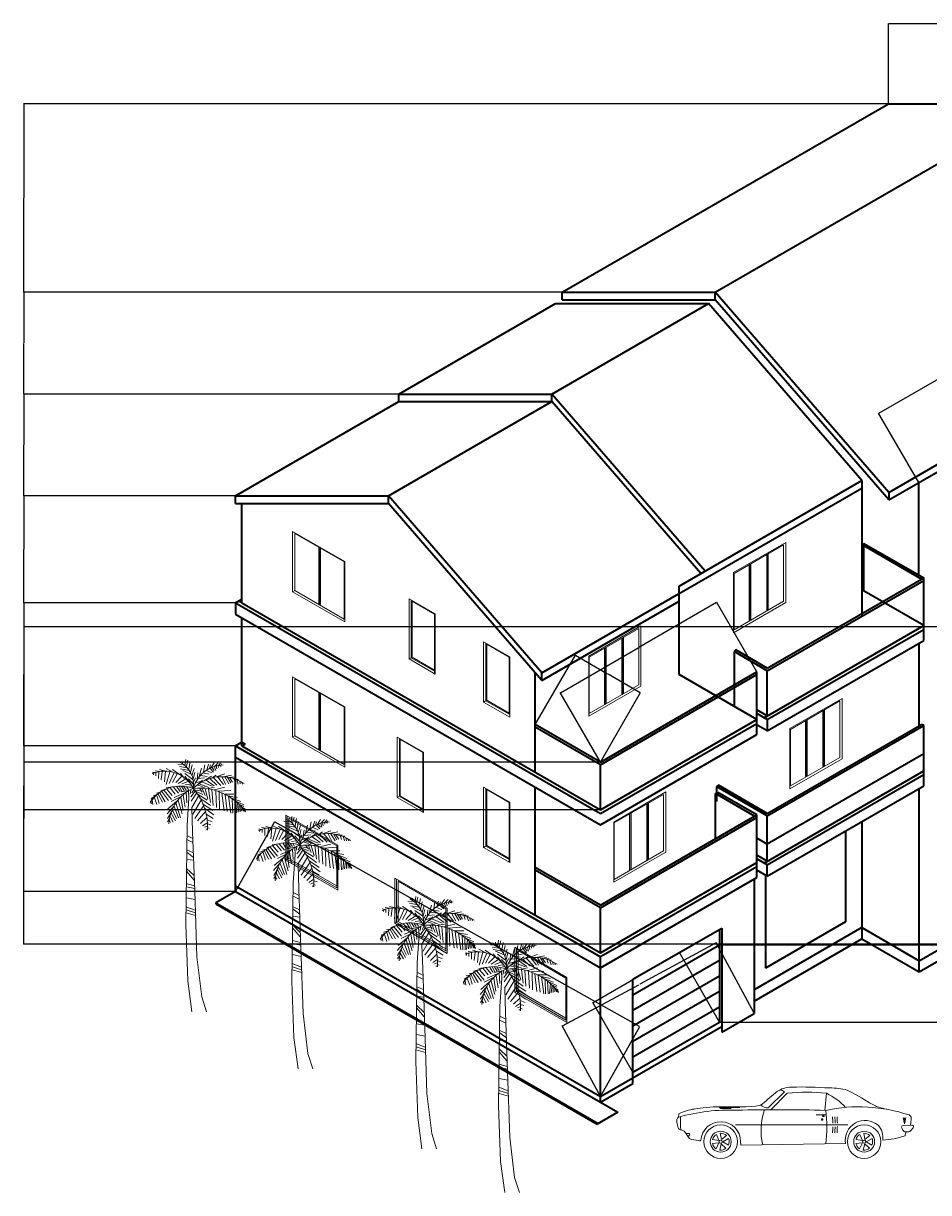
# Model space of a CAD drawing. Units: inches. Extents: x 159268 to 319465, y 115871 to 232488.
# Tile 1 of 2: x 159268 to 159989, y 115871 to 116803. Entities that reach past the tile are written whole.
import ezdxf

# ---------------------------------------------------------------- set-up
doc = ezdxf.new("R2010")
doc.units = ezdxf.units.IN
for name, color, linetype, lineweight in [('A-ANNO-DIMS', 2, 'Continuous', 18), ('A-ANNO-NPLT', 8, 'Continuous', 13), ('A-ELEV', 7, 'Continuous', 35), ('A-GLAZ', 4, 'Continuous', 18), ('C-SITE-VHCL', 8, 'Continuous', 13), ('L-PLNT', 3, 'Continuous', 13)]:
    doc.layers.add(name, color=color, linetype=linetype, lineweight=lineweight)
doc.styles.get("Standard").update_dxf_attribs({"font": 'arial.ttf'})
doc.dimstyles.get("Standard").update_dxf_attribs({"dimtxt": 0.18, "dimasz": 0.18, "dimexe": 0.18, "dimexo": 0.0625, "dimgap": 0.09, "dimtad": 0, "dimtih": 1, "dimtoh": 1, "dimdec": 4, "dimzin": 0, "dimdsep": 46, "dimtxsty": 'Standard', "dimcen": 0.09, "dimadec": 0, "dimazin": 0, "dimtfac": 1, "dimtdec": 4, "dimtofl": 0, "dimtmove": 0, "dimatfit": 3, "dimfxl": 1, "dimtolj": 1, "dimtzin": 0, "dimarcsym": 0})

# ---------------------------------------------------------------- blocks, each defined once
blk = doc.blocks.new('*U2')
for p, q in [((72.93, 40.23), (85.8, 53.18)), ((75, 38.82), (88.08, 51.97)), ((119.39, 51.91), (117.92, 38.32)), ((50.13, 41.06), (34.31, 40.98)), ((43.26, 39.85), (35.15, 39.78)), ((35.3, 40.46), (50.13, 40.62)), ((111.09, 34.73), (118.48, 34.64)), ((7.45, 19.78), (9.74, 19.8)), ((10.37, 19.19), (10.38, 18.56)), ((46.65, 26.83), (136.29, 26.77)), ((179.3, 24.35), (180.25, 22.49)), ((180.37, 26.17), (187.51, 26.41)), ((182.62, 21.14), (184.91, 21.28)), ((186.68, 22.17), (188.51, 24.37)), ((9.76, 17.93), (8.53, 17.92)), ((50.87, 13.52), (50.91, 10.52))]:
    blk.add_line(p, q)
for points in [[(35.31, 39.93), (35.3, 40.27, 0.269532), (35.14, 40.54), (34.38, 40.96, 0.575383), (34.15, 40.83), (34.15, 40.49, 0.269532), (34.32, 40.22), (35.08, 39.79, 0.575383)], [(28.49, 15.1), (33.61, 14.4), (31.65, 19.18, 0.199906)], [(34.64, 20.05), (35.56, 14.97), (39.5, 18.31, 0.199906)], [(142.85, 15.1), (147.96, 14.4), (146.01, 19.18, 0.199906)], [(148.99, 20.05), (149.91, 14.97), (153.85, 18.31, 0.199906)], [(31.31, 7.72), (33.55, 12.37), (28.4, 11.99, 0.199906)], [(39.19, 8.12), (35.46, 11.69), (34.23, 6.67, 0.199906)], [(41.25, 15.74), (36.7, 13.3), (41.09, 10.58, 0.199906)], [(145.66, 7.72), (147.9, 12.37), (142.75, 11.99, 0.199906)], [(153.54, 8.12), (149.81, 11.69), (148.59, 6.67, 0.199906)], [(155.6, 15.74), (151.06, 13.3), (155.45, 10.58, 0.199906)]]:
    blk.add_lwpolyline(points, format="xyb", close=True)
for points in [[(181.58, 27.46), (181.53, 31.95), (180.48, 32.43)], [(181.58, 27.46), (181.53, 31.95), (182.57, 32.45)], [(50.91, 10.52), (134.38, 11.83)]]:
    blk.add_lwpolyline(points)
for centre, radius in [((115.89, 31.01), 0.619), ((34.98, 13.35), 13.35), ((34.98, 13.35), 8.35), ((149.33, 13.35), 13.35), ((149.33, 13.35), 8.35), ((34.98, 13.35), 1.25), ((149.33, 13.35), 1.25)]:
    blk.add_circle(centre, radius)
for centre, radius, start, end in [((114.6, 105.09), 59.37, 237.61027, 240.97846), ((103.45, -95), 147.78, 83.81633, 95.97054), ((95.51, 3.91), 53.61, 43.27479, 63.56652), ((42.18, -111.35), 149.91, 87.83928, 105.80965), ((20.53, -3.15), 43.06, 98.53035, 116.11198), ((80.1, -1364.13), 1402.96, 88.42296, 91.3179), ((73.29, 50.49), 10.26, 230.42401, 268.00854), ((118.31, 22.51), 51.16, 161.43071, 193.23633), ((145.17, -84.88), 125.99, 71.52833, 102.12419), ((25.66, 24.94), 94.01, 351.8279, 8.16738), ((79.16, 30.11), 76.3, 177.57734, 185.52052), ((34.98, 13.35), 15.9, 0.63732, 176.34123), ((45.64, 26.83), 78.76, 0.85201, 4.65562), ((47.43, 26.85), 78.76, 0.85201, 4.65562), ((49.23, 26.87), 78.76, 0.85201, 4.65562), ((150.1, 14.36), 15.92, 49.2263, 189.1528), ((216.26, 37.76), 36.17, 188.46832, 196.53145), ((146.68, 36.98), 36.17, 344.74319, 352.80633), ((184.3, 32.25), 2.49, 357.93203, 71.52833), ((116.55, 34.7), 70.29, 353.19423, 357.93203), ((9.75, 19.18), 0.623, 0.63732, 90.63732), ((45.64, 26.83), 78.76, 355.26443, 358.86328), ((47.43, 26.85), 78.76, 355.26443, 358.86328), ((49.23, 26.87), 78.76, 355.26443, 358.86328), ((149.4, 16.55), 14.84, 352.72855, 41.66131), ((180.41, 24.92), 1.25, 91.93898, 207.10902), ((182.47, 23.63), 2.49, 207.10902, 273.46767), ((114.25, 37.03), 70.29, 344.3985, 346.93849), ((184.76, 23.76), 2.49, 273.46767, 320.16835), ((187.55, 25.16), 1.25, 320.16835, 91.93898), ((9.76, 18.55), 0.623, 270.63732, 0.63732), ((162.47, 70.82), 56.18, 271.6865, 290.2774)]:
    blk.add_arc(centre, radius, start, end)
blk.add_ellipse((116.89, 33.59), major_axis=(-0.63, -0.007), ratio=0.610043)
for points, knots in [([(11.39, 38.92), (18.06, 40.19), (30.91, 42.01), (64.77, 40.11), (70.25, 44.91), (82.35, 56.38), (99.18, 57.3), (116.06, 56.35), (133.04, 55.87), (145.24, 49.87), (153.62, 43.8), (161.17, 40.68), (164.92, 39.73), (167.29, 39.15)], [18.629823, 18.629823, 18.629823, 18.629823, 19.527405, 20.700571, 21.107983, 21.608568, 21.92336, 23.151359, 23.716171, 23.908743, 24.77794, 24.943072, 25.187755, 25.187755, 25.187755, 25.187755]), ([(19.11, 14.36), (18.99, 14.21), (18.5, 13.81), (15.35, 15), (9.19, 13.94), (7.26, 22.22), (3.01, 22.66), (1.32, 23.61), (0.64, 26.92), (-0.96, 31.49), (1.54, 32.64), (1.5, 34.06), (1.49, 34.8), (1.49, 35.06), (1.52, 35.3), (1.58, 35.51)], [16.815853, 16.815853, 16.815853, 16.815853, 16.838212, 16.885395, 17.18439, 17.479846, 17.654423, 17.670693, 17.696923, 18.016358, 18.052739, 18.140805, 18.140805, 18.140805, 18.172382, 18.172382, 18.172382, 18.172382])]:
    blk.add_open_spline(points, degree=3, knots=knots)
blk = doc.blocks.new('*U5')
for p, q in [((-6.727, 197.202), (-11.366, 197.45)), ((-7.5, 199.68), (-7.5, 197.946)), ((-5.567, 196.707), (-4.987, 201.167)), ((-4.407, 195.716), (-3.247, 200.672)), ((-2.474, 193.733), (-1.315, 199.433)), ((-1.121, 190.759), (0.232, 196.955)), ((9.317, 191.255), (10.283, 196.955)), ((11.829, 192.99), (13.182, 197.45)), ((13.956, 194.229), (14.729, 196.955)), ((15.116, 194.477), (17.822, 198.689)), ((18.015, 195.716), (20.914, 198.689)), ((19.368, 196.459), (19.948, 193.733)), ((20.914, 196.459), (21.301, 194.972)), ((21.301, 196.459), (22.847, 198.441)), ((22.074, 196.707), (23.427, 195.716)), ((23.234, 196.707), (23.62, 197.698)), ((-29.729, 190.759), (-31.469, 191.255)), ((-30.309, 190.512), (-30.695, 189.025)), ((-25.283, 191.751), (-29.342, 192.246)), ((-28.763, 190.759), (-28.763, 188.281)), ((-26.443, 191.503), (-26.636, 186.051)), ((-20.064, 191.751), (-25.863, 193.238)), ((-23.737, 191.751), (-24.51, 185.06)), ((-21.031, 191.998), (-21.804, 183.325)), ((-15.232, 191.255), (-20.644, 193.981)), ((-17.551, 191.503), (-20.451, 181.343)), ((-14.265, 190.759), (-18.131, 182.086)), ((-9.433, 189.025), (-15.618, 193.238)), ((-11.753, 189.768), (-15.425, 182.83)), ((-8.08, 188.034), (-12.912, 182.83)), ((-3.441, 194.477), (-10.013, 195.716)), ((-1.894, 192.494), (-9.24, 193.733)), ((-6.147, 186.299), (-9.24, 190.264)), ((-0.541, 189.52), (-7.307, 192.494)), ((-5.76, 190.016), (0.618, 185.308)), ((-5.76, 188.034), (-1.508, 182.582)), ((0.038, 188.281), (1.778, 193.981)), ((1.005, 185.803), (2.358, 190.759)), ((1.005, 182.582), (2.938, 186.547)), ((4.098, 185.06), (4.678, 190.512)), ((4.871, 186.051), (10.09, 186.547)), ((5.837, 187.786), (7.577, 194.229)), ((6.997, 188.529), (12.216, 187.786)), ((8.544, 190.512), (13.763, 189.52)), ((9.51, 184.317), (15.502, 188.034)), ((11.25, 192.494), (15.889, 190.512)), ((14.536, 193.981), (17.242, 191.255)), ((15.695, 186.299), (19.368, 188.777)), ((16.082, 194.972), (17.822, 192.494)), ((17.242, 186.547), (23.041, 180.599)), ((18.015, 195.468), (18.981, 192.494)), ((19.368, 187.29), (26.133, 189.768)), ((20.721, 187.042), (25.167, 181.343)), ((23.814, 187.29), (26.907, 181.343)), ((24.78, 187.538), (31.546, 188.777)), ((26.133, 187.29), (29.419, 181.838)), ((28.066, 187.29), (30.966, 182.582)), ((29.806, 186.795), (32.319, 183.078)), ((29.999, 186.795), (33.092, 187.29)), ((-21.031, 177.626), (-24.897, 176.387)), ((-15.618, 179.36), (-20.644, 178.617)), ((-20.064, 177.626), (-15.812, 172.67)), ((-17.358, 178.617), (-13.299, 173.661)), ((-15.038, 179.36), (-10.786, 174.404)), ((-12.332, 180.104), (-9.433, 175.643)), ((-4.987, 185.803), (-10.979, 182.086)), ((-10.206, 180.104), (-8.08, 175.891)), ((-8.273, 180.104), (-6.147, 176.635)), ((-3.247, 183.821), (-8.08, 181.838)), ((-6.34, 179.608), (-4.6, 177.13)), ((-1.315, 181.591), (-5.374, 181.095)), ((-4.021, 179.36), (-2.861, 177.378)), ((-2.668, 185.803), (1.198, 181.343)), ((-0.348, 180.352), (-1.894, 180.104)), ((1.585, 177.13), (0.038, 174.652)), ((1.585, 177.13), (6.61, 176.139)), ((2.938, 182.582), (6.61, 183.821)), ((4.098, 180.847), (8.35, 179.608)), ((4.871, 181.591), (8.544, 184.812)), ((5.644, 181.838), (13.569, 178.865)), ((6.224, 178.121), (8.157, 175.148)), ((7.384, 178.369), (10.476, 179.36)), ((7.77, 183.325), (16.082, 179.856)), ((8.157, 178.121), (10.476, 172.422)), ((10.476, 177.874), (12.796, 169.696)), ((11.25, 184.812), (17.628, 180.352)), ((11.829, 177.874), (18.015, 179.113)), ((13.182, 177.874), (14.729, 166.97)), ((14.536, 185.803), (19.948, 180.847)), ((15.889, 177.13), (16.855, 164.492)), ((18.015, 177.13), (26.133, 179.113)), ((32.512, 186.299), (35.218, 186.299)), ((33.479, 186.051), (34.445, 182.83)), ((35.605, 185.556), (37.151, 185.308)), ((35.798, 185.308), (36.958, 181.591)), ((38.118, 184.317), (38.504, 181.838)), ((39.857, 182.83), (40.244, 181.591)), ((-32.628, 167.961), (-33.208, 167.961)), ((-28.956, 172.174), (-32.435, 170.192)), ((-31.082, 169.944), (-32.435, 169.2)), ((-31.662, 168.705), (-31.082, 165.483)), ((-27.409, 173.413), (-30.695, 172.67)), ((-29.922, 170.687), (-27.989, 165.235)), ((-25.09, 175.148), (-28.376, 174.404)), ((-27.989, 172.422), (-26.056, 166.227)), ((-26.829, 173.661), (-23.544, 167.218)), ((-25.476, 174.652), (-21.224, 167.466)), ((-24.317, 175.891), (-18.711, 168.457)), ((-22.191, 176.635), (-16.391, 169.448)), ((-12.139, 167.961), (-19.098, 162.014)), ((-8.466, 171.678), (-16.585, 167.713)), ((-4.214, 175.148), (-14.072, 170.935)), ((-10.979, 168.457), (-7.887, 157.801)), ((-8.853, 170.935), (-7.113, 160.527)), ((-1.701, 176.882), (-8.66, 175.396)), ((-6.92, 172.917), (-5.374, 163.253)), ((-4.6, 174.9), (-4.021, 166.722)), ((-2.668, 176.387), (-2.376, 170.594)), ((-0.928, 176.882), (-1.508, 173.909)), ((2.551, 175.891), (-0.928, 171.431)), ((3.711, 174.404), (-0.541, 167.961)), ((5.257, 171.926), (-0.155, 163.005)), ((7.384, 168.705), (0.812, 157.553)), ((2.938, 175.891), (8.737, 173.413)), ((4.291, 173.909), (12.216, 168.953)), ((6.417, 170.439), (14.729, 164.492)), ((18.981, 175.891), (19.561, 163.005)), ((20.914, 175.891), (30.966, 176.635)), ((21.688, 175.396), (22.074, 161.518)), ((23.814, 174.404), (25.554, 160.279)), ((25.554, 173.661), (33.285, 173.661)), ((26.52, 173.165), (28.066, 159.784)), ((28.839, 172.174), (36.378, 170.687)), ((29.226, 171.926), (30.966, 158.545)), ((30.966, 170.687), (38.891, 167.713)), ((32.126, 169.696), (32.512, 158.545)), ((34.058, 168.705), (34.445, 158.545)), ((-32.628, 167.713), (-32.435, 165.979)), ((-14.265, 164.244), (-19.678, 158.049)), ((-16.005, 160.031), (-19.484, 154.084)), ((-16.585, 158.545), (-13.106, 152.35)), ((-15.618, 160.775), (-12.332, 154.332)), ((-14.265, 163.749), (-10.786, 154.828)), ((-12.719, 166.722), (-9.046, 154.828)), ((9.317, 164.244), (2.358, 154.332)), ((10.863, 159.784), (4.484, 152.35)), ((8.544, 165.979), (16.662, 160.527)), ((10.09, 162.51), (17.435, 157.058)), ((35.412, 167.713), (41.404, 164.988)), ((36.378, 166.474), (35.605, 158.792)), ((37.731, 165.235), (36.958, 159.288)), ((37.924, 165.235), (41.404, 163.749)), ((38.504, 164.492), (38.504, 159.536)), ((39.664, 163.253), (42.37, 161.766)), ((39.857, 162.757), (39.857, 160.031)), ((40.824, 161.766), (41.21, 160.031)), ((41.21, 161.518), (42.757, 160.279)), ((-18.131, 153.589), (-19.484, 151.606)), ((-17.938, 152.597), (-16.972, 151.111)), ((-17.358, 155.819), (-14.845, 151.358)), ((11.829, 155.075), (6.804, 150.119)), ((12.603, 151.111), (8.544, 148.385)), ((11.443, 157.553), (16.855, 154.332)), ((12.216, 153.093), (16.082, 151.606)), ((12.603, 149.872), (15.116, 149.128)), ((-4.081, 140.645), (0.753, 138.261)), ((12.216, 148.137), (10.09, 147.393)), ((12.409, 145.659), (11.056, 145.659)), ((12.409, 146.898), (13.763, 146.402)), ((-4.081, 137.547), (0.753, 135.163)), ((-4.081, 129.205), (1.124, 126.821)), ((-4.081, 127.298), (1.31, 123.246)), ((-4.081, 121.578), (1.31, 120.863)), ((-4.453, 112.283), (1.682, 105.133)), ((-4.267, 114.428), (1.682, 108.708)), ((-4.639, 102.273), (1.868, 100.604)), ((-4.453, 99.651), (2.24, 98.459)), ((-4.825, 83.921), (2.612, 81.061)), ((-4.453, 91.071), (2.426, 89.641)), ((-4.639, 81.299), (2.797, 78.916)), ((-4.639, 78.916), (2.797, 76.771))]:
    blk.add_line(p, q)
for points in [[(-2.363, 170.553), (-3.88, 148.505), (-4.988, 69.634), (-3.325, 24.869), (0, 0)], [(-0.116, 162.848), (0.554, 143.532), (2.217, 96.635), (3.88, 44.054), (7.76, 12.079), (11.64, 0)]]:
    blk.add_lwpolyline(points)
for centre, radius, start, end in [((-18.427, 181.448), 19.715, 350.285, 64.11229), ((25.595, 171.567), 25.395, 91.40319, 163.882), ((-21.738, 166.094), 25.899, 27.67115, 112.5305), ((23.687, 155.341), 32.188, 56.19272, 134.3213), ((-9.259, 151.732), 28.386, 68.38311, 147.5322), ((14.394, 148.393), 32.752, 113.7592, 177.4133), ((5.828, 132.718), 45.639, 35.98777, 95.82273), ((-32.8, 147.923), 45.309, 356.1943, 41.37848)]:
    blk.add_arc(centre, radius, start, end)
blk = doc.blocks.new('WIN-GROUND')
for p, q in [((159476.63, 116172), (159518.2, 116148)), ((159476.63, 116136), (159476.63, 116172)), ((159477.91, 116136.72), (159477.91, 116171.27)), ((159479.23, 116137.5), (159479.23, 116169.5)), ((159479.23, 116169.5), (159517.33, 116147.5)), ((159517.33, 116147.5), (159517.33, 116113.96)), ((159518.2, 116148), (159518.2, 116112)), ((159476.63, 116136), (159479.23, 116137.5)), ((159517.33, 116115.5), (159479.23, 116137.5)), ((159518.2, 116112), (159476.63, 116136)), ((159517.33, 116113.96), (159477.91, 116136.72))]:
    blk.add_line(p, q)
blk = doc.blocks.new('WIN-NARROW')
for p, q in [((159565.58, 116186), (159565.58, 116234)), ((159565.58, 116234), (159586.37, 116222)), ((159567.31, 116187), (159567.31, 116233)), ((159568.02, 116187.41), (159568.02, 116232.1)), ((159568.02, 116232.1), (159585.93, 116221.75)), ((159585.93, 116221.75), (159585.93, 116174.25)), ((159586.37, 116222), (159586.37, 116174)), ((159565.58, 116186), (159568.02, 116187.41)), ((159586.37, 116174), (159565.58, 116186)), ((159586.37, 116176), (159567.31, 116187)), ((159586.37, 116176.82), (159568.02, 116187.41))]:
    blk.add_line(p, q)
blk = doc.blocks.new('WIN-2PANE')
for p, q in [((159482.18, 116234.16), (159482.18, 116282.16)), ((159482.18, 116282.16), (159523.75, 116258.16)), ((159483.91, 116235.16), (159483.91, 116280.66)), ((159483.91, 116280.66), (159523.75, 116257.66)), ((159502.97, 116269.66), (159502.97, 116224.16)), ((159503.83, 116269.16), (159503.83, 116223.66)), ((159504.26, 116268.91), (159504.26, 116223.91)), ((159523.32, 116258.41), (159523.32, 116212.41)), ((159523.75, 116258.16), (159523.75, 116210.16)), ((159482.18, 116234.16), (159483.91, 116235.16)), ((159523.75, 116210.16), (159482.18, 116234.16)), ((159523.32, 116212.41), (159483.91, 116235.16)), ((159503.83, 116223.66), (159504.26, 116223.91))]:
    blk.add_line(p, q)
blk = doc.blocks.new('WIN-3PANE')
for p, q in [((159718.21, 116298.71), (159759.78, 116322.71)), ((159718.64, 116297.96), (159758.05, 116320.71)), ((159758.05, 116320.71), (159758.05, 116275.71)), ((159759.78, 116322.71), (159759.78, 116274.71)), ((159731.2, 116260.21), (159731.2, 116305.21)), ((159732.07, 116260.71), (159732.07, 116305.71)), ((159744.62, 116268.46), (159744.62, 116312.96)), ((159745.06, 116268.21), (159745.06, 116313.21)), ((159745.92, 116268.71), (159745.92, 116313.71)), ((159718.21, 116250.71), (159718.21, 116298.71)), ((159718.64, 116252.96), (159718.64, 116297.96)), ((159730.77, 116260.46), (159730.77, 116304.96)), ((159759.78, 116274.71), (159718.21, 116250.71)), ((159758.05, 116275.71), (159718.64, 116252.96)), ((159744.62, 116268.46), (159745.06, 116268.21)), ((159730.77, 116260.46), (159731.2, 116260.21))]:
    blk.add_line(p, q)
blk = doc.blocks.new('*D10')
at = {"layer": 'A-ANNO-DIMS', "color": 0, "lineweight": -2, "transparency": 16777216}
for p, q in [((159436.46, 116227.11), (159267.73, 116227.11)), ((159267.91, 116226.93), (159267.91, 116169.29)), ((159267.91, 116111.29), (159267.91, 116168.93)), ((159436.46, 116111.11), (159267.73, 116111.11))]:
    blk.add_line(p, q, dxfattribs=at)
at = {"layer": 'A-ANNO-DIMS', "color": 0, "transparency": 16777216}
for points in [[(159267.88, 116226.93), (159267.94, 116226.93), (159267.91, 116227.11)], [(159267.88, 116111.29), (159267.94, 116111.29), (159267.91, 116111.11)]]:
    blk.add_solid(points, dxfattribs=at)
at = {"layer": 'Defpoints', "color": 0, "transparency": 16777216}
for p in [(159267.91, 116227.11), (159436.52, 116227.11), (159436.52, 116111.11)]:
    blk.add_point(p, dxfattribs=at)
at = {"layer": 'A-ANNO-DIMS', "color": 0, "transparency": 16777216, "insert": (159267.91, 116169.11), "char_height": 0.18, "attachment_point": 5}
blk.add_mtext('\\A1;116', dxfattribs=at)
blk = doc.blocks.new('*D11')
at = {"layer": 'A-ANNO-DIMS', "color": 0, "lineweight": -2, "transparency": 16777216}
for p, q in [((159436.46, 116341.11), (159267.73, 116341.11)), ((159267.91, 116340.93), (159267.91, 116284.29)), ((159267.91, 116227.29), (159267.91, 116283.93)), ((159436.46, 116227.11), (159267.73, 116227.11))]:
    blk.add_line(p, q, dxfattribs=at)
at = {"layer": 'A-ANNO-DIMS', "color": 0, "transparency": 16777216}
for points in [[(159267.88, 116340.93), (159267.94, 116340.93), (159267.91, 116341.11)], [(159267.88, 116227.29), (159267.94, 116227.29), (159267.91, 116227.11)]]:
    blk.add_solid(points, dxfattribs=at)
at = {"layer": 'Defpoints', "color": 0, "transparency": 16777216}
for p in [(159267.91, 116341.11), (159436.52, 116341.11), (159436.52, 116227.11)]:
    blk.add_point(p, dxfattribs=at)
at = {"layer": 'A-ANNO-DIMS', "color": 0, "transparency": 16777216, "insert": (159267.91, 116284.11), "char_height": 0.18, "attachment_point": 5}
blk.add_mtext('\\A1;114', dxfattribs=at)
blk = doc.blocks.new('*D12')
at = {"layer": 'A-ANNO-DIMS', "color": 0, "lineweight": -2, "transparency": 16777216}
for p, q in [((159436.46, 116426.35), (159267.73, 116426.35)), ((159267.91, 116426.17), (159267.91, 116383.91)), ((159267.91, 116341.29), (159267.91, 116383.55)), ((159436.46, 116341.11), (159267.73, 116341.11))]:
    blk.add_line(p, q, dxfattribs=at)
at = {"layer": 'A-ANNO-DIMS', "color": 0, "transparency": 16777216}
for points in [[(159267.88, 116426.17), (159267.94, 116426.17), (159267.91, 116426.35)], [(159267.88, 116341.29), (159267.94, 116341.29), (159267.91, 116341.11)]]:
    blk.add_solid(points, dxfattribs=at)
at = {"layer": 'Defpoints', "color": 0, "transparency": 16777216}
for p in [(159267.91, 116426.35), (159436.52, 116426.35), (159436.52, 116341.11)]:
    blk.add_point(p, dxfattribs=at)
at = {"layer": 'A-ANNO-DIMS', "color": 0, "transparency": 16777216, "insert": (159267.91, 116383.73), "char_height": 0.18, "attachment_point": 5}
blk.add_mtext('\\A1;85.24', dxfattribs=at)
blk = doc.blocks.new('*D13')
at = {"layer": 'A-ANNO-DIMS', "color": 0, "lineweight": -2, "transparency": 16777216}
for p, q in [((159566.67, 116507.53), (159267.73, 116507.53)), ((159267.91, 116507.35), (159267.91, 116467.12)), ((159267.91, 116426.53), (159267.91, 116466.76)), ((159436.46, 116426.35), (159267.73, 116426.35))]:
    blk.add_line(p, q, dxfattribs=at)
at = {"layer": 'A-ANNO-DIMS', "color": 0, "transparency": 16777216}
for points in [[(159267.88, 116507.35), (159267.94, 116507.35), (159267.91, 116507.53)], [(159267.88, 116426.53), (159267.94, 116426.53), (159267.91, 116426.35)]]:
    blk.add_solid(points, dxfattribs=at)
at = {"layer": 'Defpoints', "color": 0, "transparency": 16777216}
for p in [(159267.91, 116507.53), (159566.74, 116507.53), (159436.52, 116426.35)]:
    blk.add_point(p, dxfattribs=at)
at = {"layer": 'A-ANNO-DIMS', "color": 0, "transparency": 16777216, "insert": (159267.91, 116466.94), "char_height": 0.18, "attachment_point": 5}
blk.add_mtext('\\A1;81.18', dxfattribs=at)
blk = doc.blocks.new('*D14')
at = {"layer": 'A-ANNO-DIMS', "color": 0, "lineweight": -2, "transparency": 16777216}
for p, q in [((159696.94, 116588.74), (159267.73, 116588.74)), ((159267.91, 116588.56), (159267.91, 116548.31)), ((159267.91, 116507.71), (159267.91, 116547.95)), ((159566.67, 116507.53), (159267.73, 116507.53))]:
    blk.add_line(p, q, dxfattribs=at)
at = {"layer": 'A-ANNO-DIMS', "color": 0, "transparency": 16777216}
for points in [[(159267.88, 116588.56), (159267.94, 116588.56), (159267.91, 116588.74)], [(159267.88, 116507.71), (159267.94, 116507.71), (159267.91, 116507.53)]]:
    blk.add_solid(points, dxfattribs=at)
at = {"layer": 'Defpoints', "color": 0, "transparency": 16777216}
for p in [(159267.91, 116588.74), (159697, 116588.74), (159566.74, 116507.53)]:
    blk.add_point(p, dxfattribs=at)
at = {"layer": 'A-ANNO-DIMS', "color": 0, "transparency": 16777216, "insert": (159267.91, 116548.13), "char_height": 0.18, "attachment_point": 5}
blk.add_mtext('\\A1;81.2', dxfattribs=at)
blk = doc.blocks.new('*D15')
at = {"layer": 'A-ANNO-DIMS', "color": 0, "lineweight": -2, "transparency": 16777216}
for p, q in [((159957.23, 116739.02), (159267.73, 116739.02)), ((159267.91, 116738.84), (159267.91, 116664.06)), ((159267.91, 116588.92), (159267.91, 116663.69)), ((159696.94, 116588.74), (159267.73, 116588.74))]:
    blk.add_line(p, q, dxfattribs=at)
at = {"layer": 'A-ANNO-DIMS', "color": 0, "transparency": 16777216}
for points in [[(159267.88, 116738.84), (159267.94, 116738.84), (159267.91, 116739.02)], [(159267.88, 116588.92), (159267.94, 116588.92), (159267.91, 116588.74)]]:
    blk.add_solid(points, dxfattribs=at)
at = {"layer": 'Defpoints', "color": 0, "transparency": 16777216}
for p in [(159267.91, 116739.02), (159957.3, 116739.02), (159697, 116588.74)]:
    blk.add_point(p, dxfattribs=at)
at = {"layer": 'A-ANNO-DIMS', "color": 0, "transparency": 16777216, "insert": (159267.91, 116663.88), "char_height": 0.18, "attachment_point": 5}
blk.add_mtext('\\A1;150.28', dxfattribs=at)
blk = doc.blocks.new('*D16')
at = {"layer": 'A-ANNO-DIMS', "color": 0, "lineweight": -2, "transparency": 16777216}
for p, q in [((159436.55, 116111.16), (159467.88, 116166.93)), ((159467.95, 116166.69), (159612.96, 116085.21)), ((159758.62, 116003.36), (159613.61, 116084.84)), ((159727.53, 115947.66), (159758.87, 116003.43))]:
    blk.add_line(p, q, dxfattribs=at)
at = {"layer": 'A-ANNO-DIMS', "color": 0, "transparency": 16777216}
for points in [[(159467.97, 116166.71), (159467.94, 116166.66), (159467.8, 116166.77)], [(159758.64, 116003.39), (159758.61, 116003.34), (159758.78, 116003.27)]]:
    blk.add_solid(points, dxfattribs=at)
at = {"layer": 'Defpoints', "color": 0, "transparency": 16777216}
for p in [(159436.52, 116111.11), (159758.78, 116003.27), (159727.5, 115947.61)]:
    blk.add_point(p, dxfattribs=at)
at = {"layer": 'A-ANNO-DIMS', "color": 0, "transparency": 16777216, "insert": (159613.29, 116085.02), "char_height": 0.18, "attachment_point": 5}
blk.add_mtext('\\A1;333.8', dxfattribs=at)
blk = doc.blocks.new('*D17')
at = {"layer": 'A-ANNO-DIMS', "color": 0, "lineweight": -2, "transparency": 16777216}
for p, q in [((159819.67, 116070.02), (159758.82, 116037.12)), ((159850.16, 116014), (159819.74, 116070.27)), ((159697.29, 116003.86), (159758.14, 116036.76)), ((159727.47, 115947.66), (159697.05, 116003.93))]:
    blk.add_line(p, q, dxfattribs=at)
at = {"layer": 'A-ANNO-DIMS', "color": 0, "transparency": 16777216}
for points in [[(159819.65, 116070.05), (159819.68, 116070), (159819.82, 116070.11)], [(159697.28, 116003.89), (159697.31, 116003.84), (159697.14, 116003.78)]]:
    blk.add_solid(points, dxfattribs=at)
at = {"layer": 'Defpoints', "color": 0, "transparency": 16777216}
for p in [(159819.82, 116070.11), (159850.19, 116013.94), (159727.5, 115947.61)]:
    blk.add_point(p, dxfattribs=at)
at = {"layer": 'A-ANNO-DIMS', "color": 0, "transparency": 16777216, "insert": (159758.48, 116036.94), "char_height": 0.18, "attachment_point": 5}
blk.add_mtext('\\A1;139.47', dxfattribs=at)
blk = doc.blocks.new('*D18')
at = {"layer": 'A-ANNO-DIMS', "color": 0, "lineweight": -2, "transparency": 16777216}
for p, q in [((159790.4, 116062.15), (159756.37, 116042.5)), ((159822.45, 116007), (159790.46, 116062.4)), ((159721.71, 116022.5), (159755.74, 116042.14)), ((159753.45, 115967.16), (159721.47, 116022.56))]:
    blk.add_line(p, q, dxfattribs=at)
at = {"layer": 'A-ANNO-DIMS', "color": 0, "transparency": 16777216}
for points in [[(159790.38, 116062.18), (159790.41, 116062.12), (159790.55, 116062.24)], [(159721.7, 116022.52), (159721.73, 116022.47), (159721.56, 116022.41)]]:
    blk.add_solid(points, dxfattribs=at)
at = {"layer": 'Defpoints', "color": 0, "transparency": 16777216}
for p in [(159790.55, 116062.24), (159822.48, 116006.94), (159753.48, 115967.11)]:
    blk.add_point(p, dxfattribs=at)
at = {"layer": 'A-ANNO-DIMS', "color": 0, "transparency": 16777216, "insert": (159756.06, 116042.32), "char_height": 0.18, "attachment_point": 5}
blk.add_mtext('\\A1;79.67', dxfattribs=at)
blk = doc.blocks.new('*D19')
at = {"layer": 'A-ANNO-DIMS', "color": 0, "lineweight": -2, "transparency": 16777216}
for p, q in [((159822.54, 116068.59), (160661.48, 116068.59)), ((160661.3, 116068.41), (160661.3, 116037.95)), ((160661.3, 116007.12), (160661.3, 116037.59)), ((159822.54, 116006.94), (160661.48, 116006.94))]:
    blk.add_line(p, q, dxfattribs=at)
at = {"layer": 'A-ANNO-DIMS', "color": 0, "transparency": 16777216}
for points in [[(160661.27, 116068.41), (160661.33, 116068.41), (160661.3, 116068.59)], [(160661.27, 116007.12), (160661.33, 116007.12), (160661.3, 116006.94)]]:
    blk.add_solid(points, dxfattribs=at)
at = {"layer": 'Defpoints', "color": 0, "transparency": 16777216}
for p in [(159822.48, 116068.59), (160661.3, 116068.59), (159822.48, 116006.94)]:
    blk.add_point(p, dxfattribs=at)
at = {"layer": 'A-ANNO-DIMS', "color": 0, "transparency": 16777216, "insert": (160661.3, 116037.77), "char_height": 0.18, "attachment_point": 5}
blk.add_mtext('\\A1;61.65', dxfattribs=at)
blk = doc.blocks.new('*D20')
at = {"layer": 'A-ANNO-DIMS', "color": 0, "lineweight": -2, "transparency": 16777216}
for p, q in [((160177.25, 116623.87), (160063.72, 116558.33)), ((160209.3, 116568.72), (160177.32, 116624.12)), ((159949.55, 116492.41), (160063.09, 116557.96)), ((159981.29, 116437.08), (159949.31, 116492.48))]:
    blk.add_line(p, q, dxfattribs=at)
at = {"layer": 'A-ANNO-DIMS', "color": 0, "transparency": 16777216}
for points in [[(160177.23, 116623.9), (160177.26, 116623.85), (160177.41, 116623.96)], [(159949.54, 116492.44), (159949.57, 116492.39), (159949.4, 116492.32)]]:
    blk.add_solid(points, dxfattribs=at)
at = {"layer": 'Defpoints', "color": 0, "transparency": 16777216}
for p in [(160177.41, 116623.96), (160209.33, 116568.67), (159981.32, 116437.03)]:
    blk.add_point(p, dxfattribs=at)
at = {"layer": 'A-ANNO-DIMS', "color": 0, "transparency": 16777216, "insert": (160063.4, 116558.14), "char_height": 0.18, "attachment_point": 5}
blk.add_mtext('\\A1;263.3', dxfattribs=at)
blk = doc.blocks.new('*D22')
at = {"layer": 'A-ANNO-DIMS', "color": 0, "lineweight": -2, "transparency": 16777216}
for p, q in [((160024.97, 116321.98), (159267.73, 116321.98)), ((159267.91, 116321.8), (159267.91, 116195.69)), ((159267.91, 116069.21), (159267.91, 116195.33)), ((160024.97, 116069.03), (159267.73, 116069.03))]:
    blk.add_line(p, q, dxfattribs=at)
at = {"layer": 'A-ANNO-DIMS', "color": 0, "transparency": 16777216}
for points in [[(159267.88, 116321.8), (159267.94, 116321.8), (159267.91, 116321.98)], [(159267.88, 116069.21), (159267.94, 116069.21), (159267.91, 116069.03)]]:
    blk.add_solid(points, dxfattribs=at)
at = {"layer": 'Defpoints', "color": 0, "transparency": 16777216}
for p in [(159267.91, 116321.98), (160025.03, 116321.98), (160025.03, 116069.03)]:
    blk.add_point(p, dxfattribs=at)
at = {"layer": 'A-ANNO-DIMS', "color": 0, "transparency": 16777216, "insert": (159267.91, 116195.51), "char_height": 0.18, "attachment_point": 5}
blk.add_mtext('\\A1;252.95', dxfattribs=at)
blk = doc.blocks.new('*D31')
at = {"layer": 'A-ANNO-DIMS', "color": 0, "lineweight": -2, "transparency": 16777216}
for p, q in [((159820.13, 116341.32), (159758.21, 116305.57)), ((159852.18, 116286.16), (159820.2, 116341.56)), ((159695.73, 116269.5), (159757.65, 116305.24)), ((159727.47, 116214.16), (159695.49, 116269.56))]:
    blk.add_line(p, q, dxfattribs=at)
at = {"layer": 'A-ANNO-DIMS', "color": 0, "transparency": 16777216}
for points in [[(159820.12, 116341.34), (159820.15, 116341.29), (159820.29, 116341.41)], [(159695.72, 116269.52), (159695.75, 116269.47), (159695.58, 116269.41)]]:
    blk.add_solid(points, dxfattribs=at)
at = {"layer": 'Defpoints', "color": 0, "transparency": 16777216}
for p in [(159820.29, 116341.41), (159852.21, 116286.11), (159727.5, 116214.11)]:
    blk.add_point(p, dxfattribs=at)
at = {"layer": 'A-ANNO-DIMS', "color": 0, "transparency": 16777216, "insert": (159757.93, 116305.41), "char_height": 0.18, "attachment_point": 5}
blk.add_mtext('\\A1;144', dxfattribs=at)
blk = doc.blocks.new('*D32')
at = {"layer": 'A-ANNO-DIMS', "color": 0, "lineweight": -2, "transparency": 16777216}
for p, q in [((159675.57, 116244.16), (159707.56, 116299.56)), ((159707.62, 116299.32), (159733.23, 116284.53)), ((159759.27, 116269.5), (159733.67, 116284.28)), ((159727.53, 116214.16), (159759.52, 116269.56))]:
    blk.add_line(p, q, dxfattribs=at)
at = {"layer": 'A-ANNO-DIMS', "color": 0, "transparency": 16777216}
for points in [[(159707.64, 116299.34), (159707.61, 116299.29), (159707.47, 116299.41)], [(159759.29, 116269.52), (159759.26, 116269.47), (159759.43, 116269.41)]]:
    blk.add_solid(points, dxfattribs=at)
at = {"layer": 'Defpoints', "color": 0, "transparency": 16777216}
for p in [(159759.43, 116269.41), (159675.54, 116244.11), (159727.5, 116214.11)]:
    blk.add_point(p, dxfattribs=at)
at = {"layer": 'A-ANNO-DIMS', "color": 0, "transparency": 16777216, "insert": (159733.45, 116284.41), "char_height": 0.18, "attachment_point": 5}
blk.add_mtext('\\A1;60', dxfattribs=at)
blk = doc.blocks.new('*D33')
at = {"layer": 'A-ANNO-DIMS', "color": 0, "lineweight": -2, "transparency": 16777216}
for p, q in [((159727.44, 116214.11), (159267.73, 116214.11)), ((159267.91, 116213.93), (159267.91, 116195.29)), ((159267.91, 116176.29), (159267.91, 116194.93)), ((159727.44, 116176.11), (159267.73, 116176.11))]:
    blk.add_line(p, q, dxfattribs=at)
at = {"layer": 'A-ANNO-DIMS', "color": 0, "transparency": 16777216}
for points in [[(159267.88, 116213.93), (159267.94, 116213.93), (159267.91, 116214.11)], [(159267.88, 116176.29), (159267.94, 116176.29), (159267.91, 116176.11)]]:
    blk.add_solid(points, dxfattribs=at)
at = {"layer": 'Defpoints', "color": 0, "transparency": 16777216}
for p in [(159267.91, 116214.11), (159727.5, 116214.11), (159727.5, 116176.11)]:
    blk.add_point(p, dxfattribs=at)
at = {"layer": 'A-ANNO-DIMS', "color": 0, "transparency": 16777216, "insert": (159267.91, 116195.11), "char_height": 0.18, "attachment_point": 5}
blk.add_mtext('\\A1;38', dxfattribs=at)
blk = doc.blocks.new('*D34')
at = {"layer": 'A-ANNO-DIMS', "color": 0, "lineweight": -2, "transparency": 16777216}
for p, q in [((159957.3, 116739.08), (159957.3, 116803.05)), ((159957.48, 116802.87), (160017.98, 116802.87)), ((160079.23, 116802.87), (160018.72, 116802.87)), ((160079.41, 116739.08), (160079.41, 116803.05))]:
    blk.add_line(p, q, dxfattribs=at)
at = {"layer": 'A-ANNO-DIMS', "color": 0, "transparency": 16777216}
for points in [[(159957.48, 116802.9), (159957.48, 116802.84), (159957.3, 116802.87)], [(160079.23, 116802.9), (160079.23, 116802.84), (160079.41, 116802.87)]]:
    blk.add_solid(points, dxfattribs=at)
at = {"layer": 'Defpoints', "color": 0, "transparency": 16777216}
for p in [(160079.41, 116802.87), (159957.3, 116739.02), (160079.41, 116739.02)]:
    blk.add_point(p, dxfattribs=at)
at = {"layer": 'A-ANNO-DIMS', "color": 0, "transparency": 16777216, "insert": (160018.35, 116802.87), "char_height": 0.18, "attachment_point": 5}
blk.add_mtext('\\A1;122.1', dxfattribs=at)

msp = doc.modelspace()

# ---------------------------------------------------------------- linework, layer by layer
at = {"layer": 'A-ANNO-NPLT'}
msp.add_point((159810.642, 116262.11), dxfattribs=at)
at = {"layer": 'A-ELEV'}
for p, q in [((159697, 116588.735), (159957.297, 116739.018)), ((159819.109, 116588.735), (160079.407, 116739.018)), ((159957.297, 116739.018), (160079.407, 116739.018)), ((159697, 116588.735), (159819.109, 116588.735)), ((159697, 116582.735), (159697, 116588.735)), ((159819.109, 116582.735), (159819.109, 116588.735)), ((159957.305, 116429.161), (159819.109, 116588.735)), ((159566.736, 116507.528), (159691.679, 116579.664)), ((159688.846, 116507.528), (159813.789, 116579.664)), ((159691.679, 116579.664), (159813.789, 116579.664)), ((159697, 116582.735), (159819.109, 116582.735)), ((159697, 116582.735), (159819.109, 116582.735)), ((159935.899, 116438.664), (159813.789, 116579.664)), ((159957.305, 116423.161), (159819.109, 116582.735)), ((159957.305, 116423.161), (159819.109, 116582.735)), ((159957.305, 116429.161), (160217.603, 116579.444)), ((159957.305, 116423.161), (160217.603, 116573.444)), ((159436.519, 116426.347), (159566.736, 116501.528)), ((159558.628, 116426.347), (159688.846, 116501.528)), ((159566.736, 116507.528), (159688.846, 116507.528)), ((159566.736, 116501.528), (159566.736, 116507.528)), ((159566.736, 116501.528), (159688.846, 116501.528)), ((159566.736, 116501.528), (159688.846, 116501.528)), ((159688.846, 116501.528), (159688.846, 116507.528)), ((159810.955, 116366.528), (159688.846, 116507.528)), ((159807.491, 116364.528), (159688.846, 116501.528)), ((159807.491, 116364.528), (159688.846, 116501.528)), ((159790.171, 116354.528), (159935.899, 116438.664)), ((159935.899, 116438.664), (159935.899, 116432.664)), ((159981.323, 116363.326), (159981.323, 116437.027)), ((159436.519, 116426.347), (159558.628, 116426.347)), ((159436.519, 116420.347), (159436.519, 116426.347)), ((159558.628, 116420.347), (159558.628, 116426.347)), ((159680.738, 116285.347), (159558.628, 116426.347)), ((159790.171, 116348.528), (159935.899, 116432.664)), ((159935.899, 116432.664), (159935.899, 116330.524)), ((159957.305, 116429.161), (159957.305, 116423.161)), ((159436.519, 116420.347), (159558.628, 116420.347)), ((159441.715, 116341.11), (159441.715, 116420.347)), ((159680.738, 116279.347), (159558.628, 116420.347)), ((159935.911, 116387.545), (159937.581, 116388.581)), ((159983.554, 116360.038), (159935.911, 116387.545)), ((159937.581, 116350.581), (159937.581, 116388.581)), ((159937.581, 116388.581), (159985.286, 116361.038)), ((159860.579, 116289.038), (159985.286, 116361.038)), ((159985.286, 116311.038), (159985.286, 116361.038)), ((159790.171, 116348.528), (159790.171, 116354.528)), ((159860.579, 116287.038), (159985.286, 116359.038)), ((159436.519, 116341.11), (159441.715, 116344.11)), ((159441.715, 116341.11), (159439.117, 116342.61)), ((159680.738, 116285.347), (159790.171, 116348.528)), ((159680.738, 116279.347), (159790.171, 116342.528)), ((159790.171, 116283.929), (159790.171, 116348.528)), ((159985.286, 116323.038), (159935.899, 116351.552)), ((159436.519, 116341.11), (159727.503, 116173.11)), ((159436.519, 116341.11), (159436.519, 116332.11)), ((159441.715, 116341.11), (159727.503, 116176.11)), ((159436.519, 116332.11), (159727.503, 116164.11)), ((159441.715, 116227.11), (159441.715, 116329.11)), ((159857.981, 116249.538), (159985.286, 116323.038)), ((159860.579, 116248.038), (159985.286, 116320.038)), ((159860.579, 116239.038), (159985.286, 116311.038)), ((159981.323, 116308.749), (159981.323, 116242.992)), ((159835.368, 116303.593), (159834.218, 116302.257)), ((159860.579, 116287.038), (159834.218, 116302.257)), ((159834.218, 116302.257), (159834.218, 116258.498)), ((159860.579, 116289.038), (159835.368, 116303.593)), ((159860.579, 116251.038), (159860.579, 116287.038)), ((159675.542, 116206.11), (159675.542, 116285.347)), ((159680.738, 116279.347), (159680.738, 116285.347)), ((159727.503, 116214.11), (159852.211, 116286.11)), ((159727.503, 116212.11), (159852.211, 116284.11)), ((159852.211, 116248.11), (159790.171, 116283.929)), ((159852.211, 116236.11), (159852.211, 116286.11)), ((159860.579, 116251.038), (159852.211, 116255.869)), ((159860.579, 116248.038), (159852.211, 116252.869)), ((159727.503, 116214.11), (159675.542, 116244.11)), ((159727.503, 116212.11), (159675.542, 116242.11)), ((159727.503, 116176.11), (159852.211, 116248.11)), ((159727.503, 116173.11), (159852.211, 116245.11)), ((159860.579, 116239.038), (159851.136, 116244.489)), ((159860.579, 116248.038), (159860.579, 116239.038)), ((159860.579, 116173.28), (159983.554, 116244.28)), ((159860.579, 116171.28), (159985.286, 116243.28)), ((159985.286, 116243.28), (159983.554, 116244.28)), ((159985.286, 116195.28), (159985.286, 116243.28)), ((159727.503, 116164.11), (159852.211, 116236.11)), ((159436.519, 116227.11), (159441.715, 116230.11)), ((159436.519, 116227.11), (159727.503, 116059.11)), ((159436.519, 116218.11), (159436.519, 116227.11)), ((159441.715, 116230.11), (159444.313, 116228.61)), ((159441.715, 116227.11), (159444.313, 116228.61)), ((159441.715, 116227.11), (159727.503, 116062.11)), ((159436.519, 116218.11), (159727.503, 116050.11)), ((159436.519, 116111.11), (159436.519, 116218.11)), ((159727.503, 116176.11), (159727.503, 116212.11)), ((159985.286, 116220.762), (159860.579, 116148.762)), ((159857.981, 116133.78), (159985.286, 116207.28)), ((159860.579, 116132.28), (159985.286, 116204.28)), ((159675.542, 116092.11), (159675.542, 116194.11)), ((159821.68, 116195.738), (159819.948, 116194.738)), ((159860.579, 116171.28), (159819.948, 116194.738)), ((159819.948, 116194.738), (159819.948, 116189.483)), ((159860.579, 116173.28), (159821.68, 116195.738)), ((159860.579, 116123.28), (159985.286, 116195.28)), ((159819.208, 116189.055), (159821.034, 116190.11)), ((159819.208, 116153.055), (159819.208, 116189.055)), ((159850.385, 116171.055), (159819.208, 116189.055)), ((159819.948, 116188.628), (159819.948, 116182.677)), ((159852.211, 116172.11), (159821.034, 116190.11)), ((159981.323, 116192.992), (159981.323, 116047.039)), ((159727.503, 116100.11), (159852.211, 116172.11)), ((159727.503, 116098.11), (159852.211, 116170.11)), ((159852.211, 116131.11), (159852.211, 116172.11)), ((159860.579, 116135.28), (159860.579, 116171.28)), ((159935.899, 116166.766), (159935.899, 116073.265)), ((159922.933, 116159.28), (159922.933, 116086.779)), ((159860.579, 116148.762), (159852.211, 116153.593)), ((159860.579, 116135.28), (159852.211, 116140.111)), ((159727.503, 116100.11), (159675.542, 116130.11)), ((159727.503, 116098.11), (159675.542, 116128.11)), ((159727.503, 116062.11), (159852.211, 116134.11)), ((159730.101, 116060.61), (159852.211, 116131.11)), ((159860.579, 116132.28), (159852.211, 116137.111)), ((159852.211, 116122.11), (159852.211, 116131.11)), ((159860.579, 116123.28), (159852.211, 116128.111)), ((159860.579, 116123.28), (159860.579, 116132.28)), ((159727.503, 116050.11), (159852.211, 116122.11)), ((159850.191, 116120.943), (159850.191, 116013.943)), ((159859.01, 116124.186), (159859.01, 116049.873)), ((159436.519, 116111.11), (159420.93, 116102.11)), ((159436.519, 116111.11), (159436.519, 116115.61)), ((159436.519, 116115.61), (159727.503, 115947.61)), ((159436.519, 116111.11), (159741.36, 115935.11)), ((159420.93, 116102.11), (159725.771, 115926.11)), ((159420.93, 116102.11), (159420.93, 116101.11)), ((159420.93, 116101.11), (159724.905, 115925.61)), ((159727.503, 116062.11), (159727.503, 116098.11)), ((159753.484, 116041.11), (159824.21, 116081.943)), ((159824.21, 116081.943), (159824.21, 115998.943)), ((159935.899, 116082.265), (159850.191, 116032.781)), ((159922.933, 116086.779), (159859.01, 116049.873)), ((159935.899, 116082.265), (159981.532, 116055.918)), ((159822.478, 116080.943), (159822.478, 116006.943)), ((159850.191, 116023.781), (159935.899, 116073.265)), ((159935.899, 116073.265), (159981.532, 116046.918)), ((159981.532, 116055.918), (160014.639, 116075.033)), ((159753.484, 116028.761), (159822.478, 116068.595)), ((159727.503, 116059.11), (159730.101, 116060.61)), ((159727.503, 115943.11), (159727.503, 116059.11)), ((159753.484, 116016.413), (159822.478, 116056.246)), ((159981.532, 116046.918), (160004.247, 116060.033)), ((159753.484, 116004.064), (159822.478, 116043.898)), ((159753.484, 115958.11), (159753.484, 116041.11)), ((159753.484, 115991.716), (159822.478, 116031.549)), ((159753.484, 115979.367), (159822.478, 116019.201)), ((159753.484, 115967.11), (159822.478, 116006.943)), ((159824.21, 115998.943), (159850.191, 116013.943)), ((159753.484, 115962.61), (159824.21, 116003.443)), ((159727.503, 115947.61), (159753.484, 115962.61)), ((159727.503, 115943.11), (159753.484, 115958.11)), ((159727.503, 115943.11), (159727.503, 115947.61)), ((159741.36, 115935.11), (159724.905, 115925.61))]:
    msp.add_line(p, q, dxfattribs=at)
at = {"layer": 'A-GLAZ'}
for p, q in [((159634.422, 116262.106), (159634.422, 116310.106)), ((159634.422, 116310.106), (159655.207, 116298.106)), ((159636.154, 116263.106), (159636.154, 116309.106)), ((159636.859, 116263.512), (159636.859, 116308.199)), ((159636.859, 116308.199), (159654.774, 116297.856)), ((159654.774, 116297.856), (159654.774, 116252.356)), ((159655.207, 116298.106), (159655.207, 116250.106)), ((159634.422, 116262.106), (159636.859, 116263.512)), ((159655.207, 116250.106), (159634.422, 116262.106)), ((159654.774, 116252.356), (159636.154, 116263.106)), ((159654.774, 116253.169), (159636.859, 116263.512))]:
    msp.add_line(p, q, dxfattribs=at)

# ---------------------------------------------------------------- block references
for name, p in [('WIN-2PANE', (0, 115.846)), ('WIN-3PANE', (115.456, 66.659)), ('WIN-NARROW', (9.422, 110.406)), ('WIN-3PANE', (0, 0)), ('WIN-2PANE', (0, 0)), ('WIN-3PANE', (160.326, -57.763)), ('WIN-NARROW', (0, 0)), ('WIN-NARROW', (68.84, -39.745)), ('WIN-3PANE', (19.883, -132.277)), ('WIN-GROUND', (0, 0)), ('WIN-GROUND', (87.062, -50.265)), ('WIN-GROUND', (182.599, -105.423))]:
    msp.add_blockref(name, p, dxfattribs=at)
at = {"layer": 'C-SITE-VHCL'}
msp.add_blockref('*U2', (159788.427, 115898.308), dxfattribs=at)
at = {"layer": 'L-PLNT'}
for p in [(159401.903, 116015.047), (159486.569, 115969.739), (159585.285, 115905.995), (159651.326, 115871.043)]:
    msp.add_blockref('*U5', p, dxfattribs=at)

# ---------------------------------------------------------------- dimensions: what is measured, and where the dimension line sits
at = {"layer": 'A-ANNO-DIMS'}
dim = msp.add_linear_dim(base=(160079.407, 116802.868), p1=(159957.297, 116739.018), p2=(160079.407, 116739.018), dimstyle='Standard', override={"dimdec": 1, "dimlfac": 1, "dimrnd": 0, "dimzin": 0, "dimdsep": 46, "dimlunit": 2}, dxfattribs=at)
dim.commit()
dim.dimension.update_dxf_attribs({"geometry": '*D34', "text_midpoint": (160018.352, 116802.868)})
for base, p1, p2, angle, override, picture, middle in [((159267.907, 116739.018), (159697, 116588.735), (159957.297, 116739.018), 90, {"dimdec": 2, "dimlfac": 1, "dimrnd": 0, "dimzin": 0, "dimdsep": 46, "dimlunit": 2}, '*D15', (159267.907, 116663.877)), ((160177.406, 116623.964), (159981.323, 116437.027), (160209.331, 116568.668), 30, {"dimdec": 1, "dimlfac": 1, "dimrnd": 0, "dimzin": 0, "dimdsep": 46, "dimlunit": 2}, '*D20', (160063.402, 116558.143)), ((159267.907, 116588.735), (159566.736, 116507.528), (159697, 116588.735), 90, {"dimdec": 1, "dimlfac": 1, "dimrnd": 0, "dimzin": 0, "dimdsep": 46, "dimlunit": 2}, '*D14', (159267.907, 116548.131)), ((159267.907, 116507.528), (159436.519, 116426.347), (159566.736, 116507.528), 90, {"dimdec": 2, "dimlfac": 1, "dimrnd": 0, "dimzin": 0, "dimdsep": 46, "dimlunit": 2}, '*D13', (159267.907, 116466.937)), ((159267.907, 116426.347), (159436.519, 116341.11), (159436.519, 116426.347), 90, {"dimdec": 2, "dimlfac": 1, "dimrnd": 0, "dimzin": 0, "dimdsep": 46, "dimlunit": 2}, '*D12', (159267.907, 116383.728)), ((159267.907, 116341.11), (159436.519, 116227.11), (159436.519, 116341.11), 90, {"dimdec": 0, "dimlfac": 1, "dimrnd": 0, "dimzin": 0, "dimdsep": 46, "dimlunit": 2}, '*D11', (159267.907, 116284.11)), ((159820.286, 116341.406), (159727.503, 116214.11), (159852.211, 116286.11), 30, {"dimdec": 0, "dimlfac": 1, "dimrnd": 0, "dimzin": 0, "dimdsep": 46, "dimlunit": 2}, '*D31', (159757.932, 116305.406)), ((159267.907, 116321.984), (160025.031, 116069.033), (160025.031, 116321.984), 90, {"dimdec": 2, "dimlfac": 1, "dimrnd": 0, "dimzin": 0, "dimdsep": 46, "dimlunit": 2}, '*D22', (159267.907, 116195.509)), ((159759.428, 116269.406), (159675.542, 116244.11), (159727.503, 116214.11), 330, {"dimdec": 0, "dimlfac": 1, "dimrnd": 0, "dimzin": 0, "dimdsep": 46, "dimlunit": 2}, '*D32', (159733.448, 116284.406)), ((159267.907, 116227.11), (159436.519, 116111.11), (159436.519, 116227.11), 90, {"dimdec": 0, "dimlfac": 1, "dimrnd": 0, "dimzin": 0, "dimdsep": 46, "dimlunit": 2}, '*D10', (159267.907, 116169.11)), ((159267.907, 116214.11), (159727.503, 116176.11), (159727.503, 116214.11), 90, {"dimdec": 0, "dimlfac": 1, "dimrnd": 0, "dimzin": 0, "dimdsep": 46, "dimlunit": 2}, '*D33', (159267.907, 116195.11)), ((159758.781, 116003.275), (159436.519, 116111.11), (159727.503, 115947.61), 330.668998, {"dimdec": 1, "dimlfac": 1, "dimrnd": 0, "dimzin": 0, "dimdsep": 46, "dimlunit": 2}, '*D16', (159613.288, 116085.025)), ((159819.823, 116070.11), (159727.503, 115947.61), (159850.191, 116013.943), 28.398835, {"dimdec": 2, "dimlfac": 1, "dimrnd": 0, "dimzin": 0, "dimdsep": 46, "dimlunit": 2}, '*D17', (159758.48, 116036.943)), ((160661.3, 116068.595), (159822.478, 116006.943), (159822.478, 116068.595), 90, {"dimdec": 2, "dimlfac": 1, "dimrnd": 0, "dimzin": 0, "dimdsep": 46, "dimlunit": 2}, '*D19', (160661.3, 116037.769)), ((159790.553, 116062.239), (159753.484, 115967.11), (159822.478, 116006.943), 30, {"dimdec": 2, "dimlfac": 1, "dimrnd": 0, "dimzin": 0, "dimdsep": 46, "dimlunit": 2}, '*D18', (159756.056, 116042.322))]:
    dim = msp.add_linear_dim(base=base, p1=p1, p2=p2, angle=angle, dimstyle='Standard', override=override, dxfattribs=at)
    dim.commit()
    dim.dimension.update_dxf_attribs({"geometry": picture, "text_midpoint": middle})

doc.saveas('drawing.dxf')
